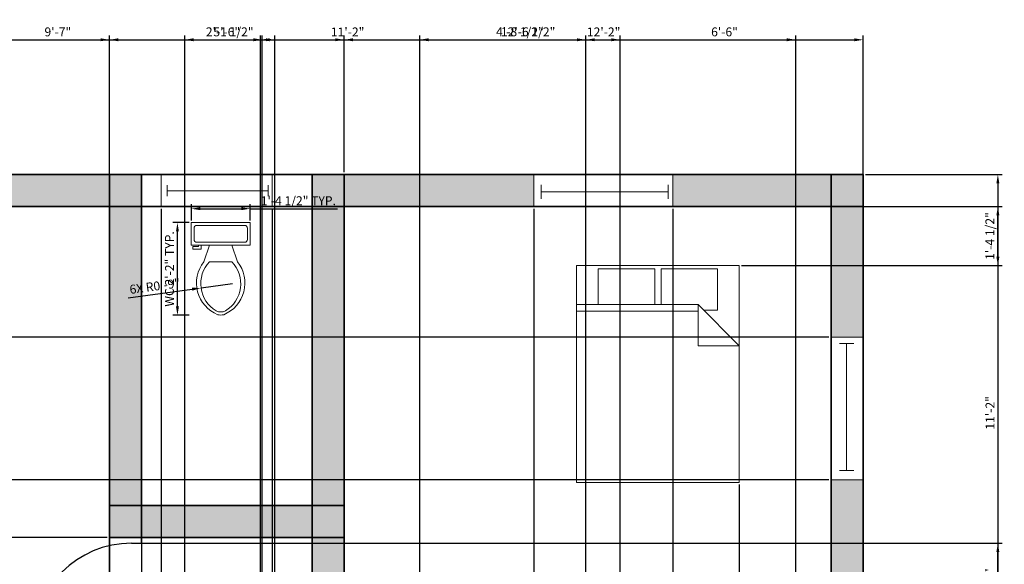
# Model space of a CAD drawing. Units: millimetres. Extents: x 2856 to 3283, y 634 to 1474.
# Tile 8 of 8: x 3006 to 3283, y 1321 to 1474. Entities that reach past the tile are written whole.
import ezdxf

# ---------------------------------------------------------------- set-up
doc = ezdxf.new("R2010")
doc.units = ezdxf.units.MM
for name, color, linetype, lineweight in [('A-ANNO-DIMS', 90, 'Continuous', 18), ('A-FLOR-FIXT', 140, 'Continuous', 18), ('A-WALL-PATT', 2, 'Continuous', 13), ('doors', 10, 'Continuous', 25), ('furniture', 140, 'Continuous', 18), ('walls', 50, 'Continuous', 35), ('windows', 30, 'Continuous', 18)]:
    doc.layers.add(name, color=color, linetype=linetype, lineweight=lineweight)
doc.styles.get("Standard").update_dxf_attribs({"font": 'arial.ttf'})
doc.dimstyles.new('ISO-25', dxfattribs={"dimtxt": 2.5, "dimasz": 2.5, "dimexe": 1.25, "dimexo": 0.625, "dimtad": 1, "dimdec": 0, "dimlunit": 3, "dimtxsty": 'Standard', "dimcen": 2.5, "dimadec": 0, "dimazin": 0, "dimtfac": 1, "dimtdec": 0, "dimtmove": 0, "dimatfit": 3, "dimfxl": 1, "dimarcsym": 0})

# ---------------------------------------------------------------- blocks, each defined once
blk = doc.blocks.new('*U3')
for p, q in [((0, 0), (0, -6)), ((40, 0), (40, -6))]:
    blk.add_line(p, q)
blk.add_lwpolyline([(0, 0), (0, 40), (1.75, 40), (1.75, 0)], close=True)
blk.add_arc((0, 0), 40, 0, 90)
blk = doc.blocks.new('*U5')
for p, q in [((0, 4), (0, 0)), ((36, 4), (36, 0)), ((0, 2), (36, 2))]:
    blk.add_line(p, q)
blk = doc.blocks.new('*U6')
for p, q in [((0, 4), (0, 0)), ((36, 4), (36, 0)), ((0, 2), (36, 2))]:
    blk.add_line(p, q)
blk = doc.blocks.new('Bed - Queen')
for p, q in [((0, -80.00003), (0, 0)), ((0, 0), (59.99999, 0)), ((59.99999, 0), (59.99999, -80.00003)), ((7.99999, -1.2), (28.79998, -1.2)), ((7.99999, -14.4), (7.99999, -1.2)), ((28.79998, -1.2), (28.79998, -14.4)), ((31.19999, -1.2), (51.99999, -1.2)), ((31.19999, -14.4), (31.19999, -1.2)), ((51.99999, -1.2), (51.99999, -16.4)), ((0, -14.4), (44.8, -14.4)), ((59.99999, -29.6), (44.8, -14.4)), ((44.8, -14.4), (44.8, -29.6)), ((44.8, -16.8), (0, -16.8)), ((51.99999, -16.4), (46.79936, -16.4)), ((44.8, -29.6), (59.99999, -29.6)), ((59.99999, -80.00003), (0, -80.00003))]:
    blk.add_line(p, q)
blk = doc.blocks.new('Toilet - top')
for p, q in [((9.5, -6), (9.5, -2)), ((-10, -8.5), (-8, -8.5)), ((-10, -9.5), (-10, -8.5)), ((-7, -9.5), (-10, -9.5)), ((-8, -8.5), (-8, -8)), ((-7, -8), (-7, -9.5)), ((-4, -8), (-6, -14)), ((4, -8), (6, -14)), ((4, -14), (-4, -14))]:
    blk.add_line(p, q)
blk.add_lwpolyline([(10.5, -8), (10.5, 0), (-10.5, 0), (-10.5, -8)], close=True)
for points in [[(-9.5, -2), (-9.5, -6)], [(8.5, -1), (-8.5, -1)], [(-8.5, -7), (8.5, -7)]]:
    blk.add_lwpolyline(points)
for centre, radius, start, end in [((-8.62, -1.88), 0.884, 81.8699, 188.1301), ((8.62, -1.88), 0.884, 351.8699, 98.1301), ((-8.62, -6.12), 0.884, 171.8699, 278.1301), ((8.62, -6.12), 0.884, 261.8699, 8.1301), ((3.52, -21.58), 12.17, 141.4691, 247.9714), ((4.2, -21.82), 11.33, 136.3677, 238.9468), ((-3.52, -21.58), 12.17, 292.0284, 38.5307), ((-4.2, -21.82), 11.33, 301.053, 43.6321), ((0, -27.88), 4, 245.7318, 294.2682), ((0, -29), 4, 254.8605, 285.1395)]:
    blk.add_arc(centre, radius, start, end)
blk = doc.blocks.new('*D20')
at = {"layer": 'A-ANNO-DIMS', "color": 0, "lineweight": -2, "transparency": 16777216}
for p, q in [((3053.58, 1417.43), (3049.05, 1417.43)), ((3050.3, 1393.88), (3050.3, 1414.93)), ((3053.58, 1391.38), (3049.05, 1391.38))]:
    blk.add_line(p, q, dxfattribs=at)
at = {"layer": 'A-ANNO-DIMS', "color": 0, "transparency": 16777216}
for points in [[(3049.88, 1414.93), (3050.72, 1414.93), (3050.3, 1417.43)], [(3049.88, 1393.88), (3050.72, 1393.88), (3050.3, 1391.38)]]:
    blk.add_solid(points, dxfattribs=at)
at = {"layer": 'Defpoints', "color": 0, "transparency": 16777216}
for p in [(3050.3, 1417.43), (3054.21, 1417.43), (3054.21, 1391.38)]:
    blk.add_point(p, dxfattribs=at)
at = {"layer": 'A-ANNO-DIMS', "color": 0, "transparency": 16777216, "insert": (3048.38, 1404.4), "char_height": 2.5, "attachment_point": 5, "rotation": 90}
blk.add_mtext('WC 2\'-2" TYP.', dxfattribs=at)
blk = doc.blocks.new('*D21')
at = {"layer": 'A-ANNO-DIMS', "color": 0, "lineweight": -2, "transparency": 16777216}
for p, q in [((3054.21, 1418.05), (3054.21, 1422.58)), ((3056.71, 1421.33), (3068.26, 1421.33)), ((3070.76, 1418.05), (3070.76, 1422.58)), ((3070.76, 1421.33), (3095.34, 1421.33))]:
    blk.add_line(p, q, dxfattribs=at)
at = {"layer": 'A-ANNO-DIMS', "color": 0, "transparency": 16777216}
for points in [[(3056.71, 1421.75), (3056.71, 1420.92), (3054.21, 1421.33)], [(3068.26, 1421.75), (3068.26, 1420.92), (3070.76, 1421.33)]]:
    blk.add_solid(points, dxfattribs=at)
at = {"layer": 'Defpoints', "color": 0, "transparency": 16777216}
for p in [(3070.76, 1421.33), (3054.21, 1417.43), (3070.76, 1417.43)]:
    blk.add_point(p, dxfattribs=at)
at = {"layer": 'A-ANNO-DIMS', "color": 0, "transparency": 16777216, "insert": (3084.3, 1423.25), "char_height": 2.5, "attachment_point": 5}
blk.add_mtext('1\'-4 1/2" TYP.', dxfattribs=at)
blk = doc.blocks.new('*D33')
at = {"layer": 'A-ANNO-DIMS', "color": 0, "lineweight": -2, "transparency": 16777216}
for p, q in [((3073.7, 1014.05), (3073.7, 1470.06)), ((3076.2, 1468.81), (3221.68, 1468.81)), ((3224.18, 1014.05), (3224.18, 1470.06))]:
    blk.add_line(p, q, dxfattribs=at)
at = {"layer": 'A-ANNO-DIMS', "color": 0, "transparency": 16777216}
for points in [[(3076.2, 1469.23), (3076.2, 1468.4), (3073.7, 1468.81)], [(3221.68, 1469.23), (3221.68, 1468.4), (3224.18, 1468.81)]]:
    blk.add_solid(points, dxfattribs=at)
at = {"layer": 'Defpoints', "color": 0, "transparency": 16777216}
for p in [(3224.18, 1468.81), (3073.7, 1013.42), (3224.18, 1013.42)]:
    blk.add_point(p, dxfattribs=at)
at = {"layer": 'A-ANNO-DIMS', "color": 0, "transparency": 16777216, "insert": (3148.94, 1470.73), "char_height": 2.5, "attachment_point": 5}
blk.add_mtext('12\'-6 1/2"', dxfattribs=at)
blk = doc.blocks.new('*D40')
at = {"layer": 'A-ANNO-DIMS', "color": 0, "lineweight": -2, "transparency": 16777216}
for p, q in [((3118.44, 913.07), (3118.44, 1470.06)), ((3120.94, 1468.81), (3172.32, 1468.81)), ((3174.82, 914.65), (3174.82, 1470.06))]:
    blk.add_line(p, q, dxfattribs=at)
at = {"layer": 'A-ANNO-DIMS', "color": 0, "transparency": 16777216}
for points in [[(3120.94, 1469.23), (3120.94, 1468.4), (3118.44, 1468.81)], [(3172.32, 1469.23), (3172.32, 1468.4), (3174.82, 1468.81)]]:
    blk.add_solid(points, dxfattribs=at)
at = {"layer": 'Defpoints', "color": 0, "transparency": 16777216}
for p in [(3174.82, 1468.81), (3174.82, 914.03), (3118.44, 912.44)]:
    blk.add_point(p, dxfattribs=at)
at = {"layer": 'A-ANNO-DIMS', "color": 0, "transparency": 16777216, "insert": (3146.63, 1470.73), "char_height": 2.5, "attachment_point": 5}
blk.add_mtext('4\'-8 1/2"', dxfattribs=at)
blk = doc.blocks.new('*D43')
at = {"layer": 'A-ANNO-DIMS', "color": 0, "lineweight": -2, "transparency": 16777216}
for p, q in [((3052.34, 800.56), (3052.34, 1470.06)), ((3054.84, 1468.81), (3075.18, 1468.81)), ((3077.68, 819.72), (3077.68, 1470.06))]:
    blk.add_line(p, q, dxfattribs=at)
at = {"layer": 'A-ANNO-DIMS', "color": 0, "transparency": 16777216}
for points in [[(3054.84, 1469.23), (3054.84, 1468.4), (3052.34, 1468.81)], [(3075.18, 1469.23), (3075.18, 1468.4), (3077.68, 1468.81)]]:
    blk.add_solid(points, dxfattribs=at)
at = {"layer": 'Defpoints', "color": 0, "transparency": 16777216}
for p in [(3077.68, 1468.81), (3077.68, 819.09), (3052.34, 799.94)]:
    blk.add_point(p, dxfattribs=at)
at = {"layer": 'A-ANNO-DIMS', "color": 0, "transparency": 16777216, "insert": (3065.01, 1470.73), "char_height": 2.5, "attachment_point": 5}
blk.add_mtext('2\'-1 1/2"', dxfattribs=at)
blk = doc.blocks.new('*D44')
at = {"layer": 'A-ANNO-DIMS', "color": 0, "lineweight": -2, "transparency": 16777216}
for p, q in [((2899.17, 1431.56), (2899.17, 1470.06)), ((2901.67, 1468.81), (3028.67, 1468.81)), ((3031.17, 1431.56), (3031.17, 1470.06))]:
    blk.add_line(p, q, dxfattribs=at)
at = {"layer": 'A-ANNO-DIMS', "color": 0, "transparency": 16777216}
for points in [[(2901.67, 1469.23), (2901.67, 1468.4), (2899.17, 1468.81)], [(3028.67, 1469.23), (3028.67, 1468.4), (3031.17, 1468.81)]]:
    blk.add_solid(points, dxfattribs=at)
at = {"layer": 'Defpoints', "color": 0, "transparency": 16777216}
for p in [(3031.17, 1468.81), (2899.17, 1430.94), (3031.17, 1430.94)]:
    blk.add_point(p, dxfattribs=at)
at = {"layer": 'A-ANNO-DIMS', "color": 0, "transparency": 16777216, "insert": (2965.17, 1470.71), "char_height": 2.5, "attachment_point": 5}
blk.add_mtext('11\'-0"', dxfattribs=at)
blk = doc.blocks.new('*D45')
at = {"layer": 'A-ANNO-DIMS', "color": 0, "lineweight": -2, "transparency": 16777216}
for p, q in [((3031.17, 1431.56), (3031.17, 1470.06)), ((3033.67, 1468.81), (3094.67, 1468.81)), ((3097.17, 1431.56), (3097.17, 1470.06))]:
    blk.add_line(p, q, dxfattribs=at)
at = {"layer": 'A-ANNO-DIMS', "color": 0, "transparency": 16777216}
for points in [[(3033.67, 1469.23), (3033.67, 1468.4), (3031.17, 1468.81)], [(3094.67, 1469.23), (3094.67, 1468.4), (3097.17, 1468.81)]]:
    blk.add_solid(points, dxfattribs=at)
at = {"layer": 'Defpoints', "color": 0, "transparency": 16777216}
for p in [(3097.17, 1468.81), (3031.17, 1430.94), (3097.17, 1430.94)]:
    blk.add_point(p, dxfattribs=at)
at = {"layer": 'A-ANNO-DIMS', "color": 0, "transparency": 16777216, "insert": (3064.17, 1470.71), "char_height": 2.5, "attachment_point": 5}
blk.add_mtext('5\'-6"', dxfattribs=at)
blk = doc.blocks.new('*D46')
at = {"layer": 'A-ANNO-DIMS', "color": 0, "lineweight": -2, "transparency": 16777216}
for p, q in [((3097.17, 1431.56), (3097.17, 1470.06)), ((3099.67, 1468.81), (3240.67, 1468.81)), ((3243.17, 1431.56), (3243.17, 1470.06))]:
    blk.add_line(p, q, dxfattribs=at)
at = {"layer": 'A-ANNO-DIMS', "color": 0, "transparency": 16777216}
for points in [[(3099.67, 1469.23), (3099.67, 1468.4), (3097.17, 1468.81)], [(3240.67, 1469.23), (3240.67, 1468.4), (3243.17, 1468.81)]]:
    blk.add_solid(points, dxfattribs=at)
at = {"layer": 'Defpoints', "color": 0, "transparency": 16777216}
for p in [(3243.17, 1468.81), (3097.17, 1430.94), (3243.17, 1430.94)]:
    blk.add_point(p, dxfattribs=at)
at = {"layer": 'A-ANNO-DIMS', "color": 0, "transparency": 16777216, "insert": (3170.17, 1470.69), "char_height": 2.5, "attachment_point": 5}
blk.add_mtext('12\'-2"', dxfattribs=at)
blk = doc.blocks.new('*D47')
at = {"layer": 'A-ANNO-DIMS', "color": 0, "lineweight": -2, "transparency": 16777216}
for p, q in [((3243.8, 1430.94), (3282.3, 1430.94)), ((3281.05, 1428.44), (3281.05, 1299.44)), ((3243.8, 1296.94), (3282.3, 1296.94))]:
    blk.add_line(p, q, dxfattribs=at)
at = {"layer": 'A-ANNO-DIMS', "color": 0, "transparency": 16777216}
for points in [[(3280.63, 1428.44), (3281.47, 1428.44), (3281.05, 1430.94)], [(3280.63, 1299.44), (3281.47, 1299.44), (3281.05, 1296.94)]]:
    blk.add_solid(points, dxfattribs=at)
at = {"layer": 'Defpoints', "color": 0, "transparency": 16777216}
for p in [(3243.17, 1430.94), (3243.17, 1296.94), (3281.05, 1296.94)]:
    blk.add_point(p, dxfattribs=at)
at = {"layer": 'A-ANNO-DIMS', "color": 0, "transparency": 16777216, "insert": (3279.17, 1363.94), "char_height": 2.5, "attachment_point": 5, "rotation": 90}
blk.add_mtext('11\'-2"', dxfattribs=at)
blk = doc.blocks.new('*D48')
at = {"layer": 'A-ANNO-DIMS', "color": 0, "lineweight": -2, "transparency": 16777216}
for p, q in [((3030.55, 1430.94), (2860.05, 1430.94)), ((2861.3, 1428.44), (2861.3, 1331.44)), ((3030.55, 1328.94), (2860.05, 1328.94))]:
    blk.add_line(p, q, dxfattribs=at)
at = {"layer": 'A-ANNO-DIMS', "color": 0, "transparency": 16777216}
for points in [[(2860.88, 1428.44), (2861.72, 1428.44), (2861.3, 1430.94)], [(2860.88, 1331.44), (2861.72, 1331.44), (2861.3, 1328.94)]]:
    blk.add_solid(points, dxfattribs=at)
at = {"layer": 'Defpoints', "color": 0, "transparency": 16777216}
for p in [(3031.17, 1430.94), (2861.3, 1328.94), (3031.17, 1328.94)]:
    blk.add_point(p, dxfattribs=at)
at = {"layer": 'A-ANNO-DIMS', "color": 0, "transparency": 16777216, "insert": (2859.4, 1379.94), "char_height": 2.5, "attachment_point": 5, "rotation": 90}
blk.add_mtext('8\'-6"', dxfattribs=at)
blk = doc.blocks.new('*D50')
at = {"layer": 'A-ANNO-DIMS', "color": 0, "lineweight": -2, "transparency": 16777216}
for p, q in [((3031.17, 1166.56), (3031.17, 1470.06)), ((3033.67, 1468.81), (3162.67, 1468.81)), ((3165.17, 1157.56), (3165.17, 1470.06))]:
    blk.add_line(p, q, dxfattribs=at)
at = {"layer": 'A-ANNO-DIMS', "color": 0, "transparency": 16777216}
for points in [[(3033.67, 1469.23), (3033.67, 1468.4), (3031.17, 1468.81)], [(3162.67, 1469.23), (3162.67, 1468.4), (3165.17, 1468.81)]]:
    blk.add_solid(points, dxfattribs=at)
at = {"layer": 'Defpoints', "color": 0, "transparency": 16777216}
for p in [(3165.17, 1468.81), (3031.17, 1165.94), (3165.17, 1156.94)]:
    blk.add_point(p, dxfattribs=at)
at = {"layer": 'A-ANNO-DIMS', "color": 0, "transparency": 16777216, "insert": (3098.17, 1470.69), "char_height": 2.5, "attachment_point": 5}
blk.add_mtext('11\'-2"', dxfattribs=at)
blk = doc.blocks.new('*D51')
at = {"layer": 'A-ANNO-DIMS', "color": 0, "lineweight": -2, "transparency": 16777216}
for p, q in [((3165.17, 1223.56), (3165.17, 1470.06)), ((3167.67, 1468.81), (3240.67, 1468.81)), ((3243.17, 1223.56), (3243.17, 1470.06))]:
    blk.add_line(p, q, dxfattribs=at)
at = {"layer": 'A-ANNO-DIMS', "color": 0, "transparency": 16777216}
for points in [[(3167.67, 1469.23), (3167.67, 1468.4), (3165.17, 1468.81)], [(3240.67, 1469.23), (3240.67, 1468.4), (3243.17, 1468.81)]]:
    blk.add_solid(points, dxfattribs=at)
at = {"layer": 'Defpoints', "color": 0, "transparency": 16777216}
for p in [(3243.17, 1468.81), (3165.17, 1222.94), (3243.17, 1222.94)]:
    blk.add_point(p, dxfattribs=at)
at = {"layer": 'A-ANNO-DIMS', "color": 0, "transparency": 16777216, "insert": (3204.17, 1470.71), "char_height": 2.5, "attachment_point": 5}
blk.add_mtext('6\'-6"', dxfattribs=at)
blk = doc.blocks.new('*D59')
at = {"layer": 'A-ANNO-DIMS', "color": 0, "lineweight": -2, "transparency": 16777216}
for p, q in [((2959.17, 1117.56), (2959.17, 1470.06)), ((2961.67, 1468.81), (3071.67, 1468.81)), ((3074.17, 1117.56), (3074.17, 1470.06))]:
    blk.add_line(p, q, dxfattribs=at)
at = {"layer": 'A-ANNO-DIMS', "color": 0, "transparency": 16777216}
for points in [[(2961.67, 1469.23), (2961.67, 1468.4), (2959.17, 1468.81)], [(3071.67, 1469.23), (3071.67, 1468.4), (3074.17, 1468.81)]]:
    blk.add_solid(points, dxfattribs=at)
at = {"layer": 'Defpoints', "color": 0, "transparency": 16777216}
for p in [(3074.17, 1468.81), (2959.17, 1116.94), (3074.17, 1116.94)]:
    blk.add_point(p, dxfattribs=at)
at = {"layer": 'A-ANNO-DIMS', "color": 0, "transparency": 16777216, "insert": (3016.67, 1470.71), "char_height": 2.5, "attachment_point": 5}
blk.add_mtext('9\'-7"', dxfattribs=at)
blk = doc.blocks.new('*D61')
at = {"layer": 'A-ANNO-DIMS', "color": 0, "lineweight": -2, "transparency": 16777216}
for p, q in [((3031.17, 1430.31), (3031.17, 634.81)), ((3040.17, 1430.31), (3040.17, 634.81)), ((3033.67, 636.06), (3037.67, 636.06))]:
    blk.add_line(p, q, dxfattribs=at)
at = {"layer": 'A-ANNO-DIMS', "color": 0, "transparency": 16777216}
for points in [[(3033.67, 636.48), (3033.67, 635.65), (3031.17, 636.06)], [(3037.67, 636.48), (3037.67, 635.65), (3040.17, 636.06)]]:
    blk.add_solid(points, dxfattribs=at)
at = {"layer": 'Defpoints', "color": 0, "transparency": 16777216}
for p in [(3031.17, 1430.94), (3040.17, 1430.94), (3040.17, 636.06)]:
    blk.add_point(p, dxfattribs=at)
at = {"layer": 'A-ANNO-DIMS', "color": 0, "transparency": 16777216, "insert": (3035.67, 637.96), "char_height": 2.5, "attachment_point": 5}
blk.add_mtext('0\'-9"', dxfattribs=at)
blk = doc.blocks.new('*D68')
at = {"layer": 'A-ANNO-DIMS', "color": 0, "lineweight": -2, "transparency": 16777216}
for p, q in [((3040.8, 1327.29), (3282.3, 1327.29)), ((3281.05, 1302.28), (3281.05, 1324.79)), ((3040.8, 1299.78), (3282.3, 1299.78))]:
    blk.add_line(p, q, dxfattribs=at)
at = {"layer": 'A-ANNO-DIMS', "color": 0, "transparency": 16777216}
for points in [[(3280.63, 1324.79), (3281.47, 1324.79), (3281.05, 1327.29)], [(3280.63, 1302.28), (3281.47, 1302.28), (3281.05, 1299.78)]]:
    blk.add_solid(points, dxfattribs=at)
at = {"layer": 'Defpoints', "color": 0, "transparency": 16777216}
for p in [(3040.17, 1327.29), (3281.05, 1327.29), (3040.17, 1299.78)]:
    blk.add_point(p, dxfattribs=at)
at = {"layer": 'A-ANNO-DIMS', "color": 0, "transparency": 16777216, "insert": (3279.13, 1313.53), "char_height": 2.5, "attachment_point": 5, "rotation": 90}
blk.add_mtext('2\'-3 1/2"', dxfattribs=at)
blk = doc.blocks.new('*D70')
at = {"layer": 'A-ANNO-DIMS', "color": 0, "lineweight": -2, "transparency": 16777216}
for p, q in [((3045.69, 1421.31), (3045.69, 634.81)), ((3076.97, 1421.31), (3076.97, 634.81)), ((3048.19, 636.06), (3074.47, 636.06))]:
    blk.add_line(p, q, dxfattribs=at)
at = {"layer": 'A-ANNO-DIMS', "color": 0, "transparency": 16777216}
for points in [[(3048.19, 636.48), (3048.19, 635.65), (3045.69, 636.06)], [(3074.47, 636.48), (3074.47, 635.65), (3076.97, 636.06)]]:
    blk.add_solid(points, dxfattribs=at)
at = {"layer": 'Defpoints', "color": 0, "transparency": 16777216}
for p in [(3045.69, 1421.94), (3076.97, 1421.94), (3076.97, 636.06)]:
    blk.add_point(p, dxfattribs=at)
at = {"layer": 'A-ANNO-DIMS', "color": 0, "transparency": 16777216, "insert": (3061.33, 637.98), "char_height": 2.5, "attachment_point": 5}
blk.add_mtext('2\'-7 1/2"', dxfattribs=at)
blk = doc.blocks.new('*D71')
at = {"layer": 'A-ANNO-DIMS', "color": 0, "lineweight": -2, "transparency": 16777216}
for p, q in [((3150.5, 1421.31), (3150.5, 634.81)), ((3189.65, 1421.31), (3189.65, 634.81)), ((3153, 636.06), (3187.15, 636.06))]:
    blk.add_line(p, q, dxfattribs=at)
at = {"layer": 'A-ANNO-DIMS', "color": 0, "transparency": 16777216}
for points in [[(3153, 636.48), (3153, 635.65), (3150.5, 636.06)], [(3187.15, 636.48), (3187.15, 635.65), (3189.65, 636.06)]]:
    blk.add_solid(points, dxfattribs=at)
at = {"layer": 'Defpoints', "color": 0, "transparency": 16777216}
for p in [(3150.5, 1421.94), (3189.65, 1421.94), (3189.65, 636.06)]:
    blk.add_point(p, dxfattribs=at)
at = {"layer": 'A-ANNO-DIMS', "color": 0, "transparency": 16777216, "insert": (3170.07, 637.97), "char_height": 2.5, "attachment_point": 5}
blk.add_mtext('3\'-3"', dxfattribs=at)
blk = doc.blocks.new('*D72')
at = {"layer": 'A-ANNO-DIMS', "color": 0, "lineweight": -2, "transparency": 16777216}
for p, q in [((3233.55, 1385.21), (2860.05, 1385.21)), ((2861.3, 1347.66), (2861.3, 1382.71)), ((3233.55, 1345.16), (2860.05, 1345.16))]:
    blk.add_line(p, q, dxfattribs=at)
at = {"layer": 'A-ANNO-DIMS', "color": 0, "transparency": 16777216}
for points in [[(2860.88, 1382.71), (2861.72, 1382.71), (2861.3, 1385.21)], [(2860.88, 1347.66), (2861.72, 1347.66), (2861.3, 1345.16)]]:
    blk.add_solid(points, dxfattribs=at)
at = {"layer": 'Defpoints', "color": 0, "transparency": 16777216}
for p in [(2861.3, 1385.21), (3234.17, 1385.21), (3234.17, 1345.16)]:
    blk.add_point(p, dxfattribs=at)
at = {"layer": 'A-ANNO-DIMS', "color": 0, "transparency": 16777216, "insert": (2859.4, 1365.19), "char_height": 2.5, "attachment_point": 5, "rotation": 90}
blk.add_mtext('3\'-4"', dxfattribs=at)
blk = doc.blocks.new('*D77')
at = {"layer": 'A-ANNO-DIMS', "color": 0, "lineweight": -2, "transparency": 16777216}
for p, q in [((3097.17, 1430.31), (3097.17, 634.81)), ((3150.5, 1421.31), (3150.5, 634.81)), ((3099.67, 636.06), (3148, 636.06))]:
    blk.add_line(p, q, dxfattribs=at)
at = {"layer": 'A-ANNO-DIMS', "color": 0, "transparency": 16777216}
for points in [[(3099.67, 636.48), (3099.67, 635.65), (3097.17, 636.06)], [(3148, 636.48), (3148, 635.65), (3150.5, 636.06)]]:
    blk.add_solid(points, dxfattribs=at)
at = {"layer": 'Defpoints', "color": 0, "transparency": 16777216}
for p in [(3097.17, 1430.94), (3150.5, 1421.94), (3150.5, 636.06)]:
    blk.add_point(p, dxfattribs=at)
at = {"layer": 'A-ANNO-DIMS', "color": 0, "transparency": 16777216, "insert": (3123.84, 637.98), "char_height": 2.5, "attachment_point": 5}
blk.add_mtext('4\'-5 1/2"', dxfattribs=at)
blk = doc.blocks.new('*D78')
at = {"layer": 'A-ANNO-DIMS', "color": 0, "lineweight": -2, "transparency": 16777216}
for p, q in [((3233.55, 1430.94), (2860.05, 1430.94)), ((2861.3, 1387.71), (2861.3, 1428.44)), ((3233.55, 1385.21), (2860.05, 1385.21))]:
    blk.add_line(p, q, dxfattribs=at)
at = {"layer": 'A-ANNO-DIMS', "color": 0, "transparency": 16777216}
for points in [[(2860.88, 1428.44), (2861.72, 1428.44), (2861.3, 1430.94)], [(2860.88, 1387.71), (2861.72, 1387.71), (2861.3, 1385.21)]]:
    blk.add_solid(points, dxfattribs=at)
at = {"layer": 'Defpoints', "color": 0, "transparency": 16777216}
for p in [(2861.3, 1430.94), (3234.17, 1430.94), (3234.17, 1385.21)]:
    blk.add_point(p, dxfattribs=at)
at = {"layer": 'A-ANNO-DIMS', "color": 0, "transparency": 16777216, "insert": (2859.38, 1408.08), "char_height": 2.5, "attachment_point": 5, "rotation": 90}
blk.add_mtext('3\'-9 1/2"', dxfattribs=at)
blk = doc.blocks.new('*D92')
at = {"layer": 'A-ANNO-DIMS', "color": 0, "lineweight": -2, "transparency": 16777216}
for p, q in [((3208.3, 1343.77), (3208.3, 634.81)), ((3234.17, 1344.54), (3234.17, 634.81)), ((3210.8, 636.06), (3231.67, 636.06))]:
    blk.add_line(p, q, dxfattribs=at)
at = {"layer": 'A-ANNO-DIMS', "color": 0, "transparency": 16777216}
for points in [[(3210.8, 636.48), (3210.8, 635.65), (3208.3, 636.06)], [(3231.67, 636.48), (3231.67, 635.65), (3234.17, 636.06)]]:
    blk.add_solid(points, dxfattribs=at)
at = {"layer": 'Defpoints', "color": 0, "transparency": 16777216}
for p in [(3208.3, 1344.39), (3234.17, 1345.16), (3234.17, 636.06)]:
    blk.add_point(p, dxfattribs=at)
at = {"layer": 'A-ANNO-DIMS', "color": 0, "transparency": 16777216, "insert": (3221.24, 637.94), "char_height": 2.5, "attachment_point": 5}
blk.add_mtext('2\'-2"', dxfattribs=at)
blk = doc.blocks.new('*D93')
at = {"layer": 'A-ANNO-DIMS', "color": 0, "lineweight": -2, "transparency": 16777216}
for p, q in [((3190.27, 1421.94), (3282.3, 1421.94)), ((3281.05, 1407.85), (3281.05, 1419.44)), ((3208.93, 1405.35), (3282.3, 1405.35))]:
    blk.add_line(p, q, dxfattribs=at)
at = {"layer": 'A-ANNO-DIMS', "color": 0, "transparency": 16777216}
for points in [[(3280.63, 1419.44), (3281.47, 1419.44), (3281.05, 1421.94)], [(3280.63, 1407.85), (3281.47, 1407.85), (3281.05, 1405.35)]]:
    blk.add_solid(points, dxfattribs=at)
at = {"layer": 'Defpoints', "color": 0, "transparency": 16777216}
for p in [(3189.65, 1421.94), (3281.05, 1421.94), (3208.3, 1405.35)]:
    blk.add_point(p, dxfattribs=at)
at = {"layer": 'A-ANNO-DIMS', "color": 0, "transparency": 16777216, "insert": (3279.13, 1413.65), "char_height": 2.5, "attachment_point": 5, "rotation": 90}
blk.add_mtext('1\'-4 1/2"', dxfattribs=at)
blk = doc.blocks.new('*D98')
at = {"layer": 'A-ANNO-DIMS', "color": 0, "lineweight": -2, "transparency": 16777216}
for p, q in [((3088.17, 1430.31), (3088.17, 634.81)), ((3076.97, 1421.31), (3076.97, 634.81)), ((3079.47, 636.06), (3085.67, 636.06))]:
    blk.add_line(p, q, dxfattribs=at)
at = {"layer": 'A-ANNO-DIMS', "color": 0, "transparency": 16777216}
for points in [[(3079.47, 636.48), (3079.47, 635.65), (3076.97, 636.06)], [(3085.67, 636.48), (3085.67, 635.65), (3088.17, 636.06)]]:
    blk.add_solid(points, dxfattribs=at)
at = {"layer": 'Defpoints', "color": 0, "transparency": 16777216}
for p in [(3088.17, 1430.94), (3076.97, 1421.94), (3088.17, 636.06)]:
    blk.add_point(p, dxfattribs=at)
at = {"layer": 'A-ANNO-DIMS', "color": 0, "transparency": 16777216, "insert": (3082.57, 637.96), "char_height": 2.5, "attachment_point": 5}
blk.add_mtext('0\'-11"', dxfattribs=at)
blk = doc.blocks.new('*D102')
at = {"layer": 'A-ANNO-DIMS', "color": 0, "lineweight": -2, "transparency": 16777216}
for p, q in [((3036.45, 1396.29), (3054.47, 1398.71)), ((3065.79, 1400.23), (3056.94, 1399.04))]:
    blk.add_line(p, q, dxfattribs=at)
at = {"layer": 'A-ANNO-DIMS', "color": 0, "transparency": 16777216}
blk.add_solid([(3054.41, 1399.12), (3054.52, 1398.3), (3056.94, 1399.04)], dxfattribs=at)
at = {"layer": 'Defpoints', "color": 0, "transparency": 16777216}
for p in [(3056.94, 1399.04), (3065.79, 1400.23)]:
    blk.add_point(p, dxfattribs=at)
at = {"layer": 'A-ANNO-DIMS', "color": 0, "transparency": 16777216, "insert": (3043.97, 1399.22), "char_height": 2.5, "attachment_point": 5, "rotation": 7.6594}
blk.add_mtext('6X R0\'-9"', dxfattribs=at)

msp = doc.modelspace()

# ---------------------------------------------------------------- hatches: boundary and pattern name
at = {"layer": 'A-WALL-PATT'}
h = msp.add_hatch(color=256, dxfattribs=at)
h.dxf.hatch_style = 1
h.paths.add_polyline_path([(2908.17, 1430.94), (2899.17, 1430.94), (2899.17, 1421.94), (2908.17, 1421.94)])
h.paths.add_polyline_path([(2908.17, 1421.94), (2899.17, 1421.94), (2899.17, 1296.94), (2908.17, 1296.94)])
h.paths.add_polyline_path([(2940.27, 1430.94), (2908.17, 1430.94), (2908.17, 1421.94), (2940.27, 1421.94)])
h.paths.add_polyline_path([(3031.17, 1430.94), (2982.35, 1430.94), (2982.35, 1421.94), (3031.17, 1421.94)])
h.paths.add_polyline_path([(3150.5, 1430.94), (3097.17, 1430.94), (3097.17, 1421.94), (3150.5, 1421.94)])
h.paths.add_polyline_path([(3097.17, 1430.94), (3088.17, 1430.94), (3088.17, 1421.94), (3097.17, 1421.94)])
h.paths.add_polyline_path([(3097.17, 1421.94), (3088.17, 1421.94), (3088.17, 1337.94), (3097.17, 1337.94)])
h.paths.add_polyline_path([(3088.17, 1337.94), (3040.17, 1337.94), (3040.17, 1328.94), (3088.17, 1328.94)])
h.paths.add_polyline_path([(3097.17, 1337.94), (3088.17, 1337.94), (3088.17, 1328.94), (3097.17, 1328.94)])
h.paths.add_polyline_path([(3097.17, 1328.94), (3088.17, 1328.94), (3088.17, 1296.94), (3097.17, 1296.94)])
h.paths.add_polyline_path([(3097.17, 1296.94), (3088.17, 1296.94), (3088.17, 1287.94), (3097.17, 1287.94)])
h.paths.add_polyline_path([(3040.17, 1421.94), (3031.17, 1421.94), (3031.17, 1337.94), (3040.17, 1337.94)])
h.paths.add_polyline_path([(3040.17, 1337.94), (3031.17, 1337.94), (3031.17, 1328.94), (3040.17, 1328.94)])
h.paths.add_polyline_path([(3040.17, 1430.94), (3031.17, 1430.94), (3031.17, 1421.94), (3040.17, 1421.94)])
h.paths.add_polyline_path([(3243.17, 1421.94), (3234.17, 1421.94), (3234.17, 1385.21), (3243.17, 1385.21)])
h.paths.add_polyline_path([(3243.17, 1430.94), (3234.17, 1430.94), (3234.17, 1421.94), (3243.17, 1421.94)])
h.paths.add_polyline_path([(3234.17, 1430.94), (3189.65, 1430.94), (3189.65, 1421.94), (3234.17, 1421.94)])
h.paths.add_polyline_path([(3243.17, 1345.16), (3234.17, 1345.16), (3234.17, 1296.94), (3243.17, 1296.94)])
h.paths.add_polyline_path([(3234.17, 1296.94), (3128.45, 1296.94, -0.06768), (3129.44, 1289.59), (3129.44, 1287.94), (3234.17, 1287.94)])
h.paths.add_polyline_path([(3031.17, 1296.94), (2908.17, 1296.94), (2908.17, 1287.94), (3031.17, 1287.94)])
h.paths.add_polyline_path([(3040.17, 1296.94), (3031.17, 1296.94), (3031.17, 1287.94), (3040.17, 1287.94)])
h.paths.add_polyline_path([(2908.17, 1296.94), (2899.17, 1296.94), (2899.17, 1287.94), (2908.17, 1287.94)])
h.paths.add_polyline_path([(2908.17, 1287.94), (2899.17, 1287.94), (2899.17, 1235.12), (2908.17, 1235.12)])
h.paths.add_polyline_path([(3040.17, 1287.94), (3031.17, 1287.94), (3031.17, 1165.94), (3040.17, 1165.94)])
h.paths.add_polyline_path([(3165.17, 1165.94), (3040.17, 1165.94), (3040.17, 1156.94), (3165.17, 1156.94)])
h.paths.add_polyline_path([(3040.17, 1165.94), (3031.17, 1165.94), (3031.17, 1156.94), (3040.17, 1156.94)])
h.paths.add_polyline_path([(3040.17, 1156.94), (3031.17, 1156.94), (3031.17, 1147.75, -0.068303), (3038.59, 1148.77), (3040.17, 1148.77)])
h.paths.add_polyline_path([(3174.17, 1197.55), (3166.11, 1197.55), (3165.17, 1197.55), (3165.17, 1165.94), (3174.17, 1165.94)])
h.paths.add_polyline_path([(3174.17, 1165.94), (3165.17, 1165.94), (3165.17, 1156.94), (3174.17, 1156.94)])
h.paths.add_polyline_path([(3234.17, 1165.94), (3174.17, 1165.94), (3174.17, 1156.94), (3234.17, 1156.94)])
h.paths.add_polyline_path([(3243.17, 1165.94), (3234.17, 1165.94), (3234.17, 1156.94), (3243.17, 1156.94)])
h.paths.add_polyline_path([(3243.17, 1172.31), (3234.17, 1172.31), (3234.17, 1165.94), (3243.17, 1165.94)])
h.paths.add_polyline_path([(3243.17, 1222.94), (3234.17, 1222.94), (3234.17, 1213.94), (3243.17, 1213.94)])
h.paths.add_polyline_path([(3234.17, 1222.94), (3174.17, 1222.94), (3174.17, 1213.94), (3234.17, 1213.94)])
h.paths.add_polyline_path([(3174.17, 1222.94), (3165.17, 1222.94), (3165.17, 1213.94), (3174.17, 1213.94)])
h.paths.add_polyline_path([(3174.17, 1270.54, -0.139319), (3166.75, 1268.43), (3165.17, 1268.43), (3165.17, 1222.94), (3174.17, 1222.94)])
h.paths.add_polyline_path([(3243.17, 1243.94), (3234.17, 1243.94), (3234.17, 1222.94), (3243.17, 1222.94)])
h.paths.add_polyline_path([(3243.17, 1213.94), (3234.17, 1213.94), (3234.17, 1203.68), (3243.17, 1203.68)])
h.paths.add_polyline_path([(3174.17, 1213.94), (3165.17, 1213.94), (3165.17, 1210.62), (3166.11, 1210.62, -0.16772), (3174.17, 1207.84)])
h.paths.add_polyline_path([(3243.17, 1296.94), (3234.17, 1296.94), (3234.17, 1287.94), (3243.17, 1287.94)])
h.paths.add_polyline_path([(3243.17, 1287.94), (3234.17, 1287.94), (3234.17, 1276.76), (3243.17, 1276.76)])
h.paths.add_polyline_path([(3174.17, 1287.94), (3165.17, 1287.94), (3165.17, 1282.56), (3166.75, 1282.56), (3174.17, 1282.56)])
h.paths.add_polyline_path([(2908.17, 1190.69), (2899.17, 1190.69), (2899.17, 1116.94), (2908.17, 1116.94)])
h.paths.add_polyline_path([(2908.17, 1107.94), (2899.17, 1107.94), (2899.17, 1058.94), (2908.17, 1058.94)])
h.paths.add_polyline_path([(2908.17, 1116.94), (2899.17, 1116.94), (2899.17, 1107.94), (2908.17, 1107.94)])
h.paths.add_polyline_path([(2959.17, 1107.94), (2950.17, 1107.94), (2950.17, 1058.94), (2959.17, 1058.94)])
h.paths.add_polyline_path([(2959.17, 1116.94), (2950.17, 1116.94), (2950.17, 1107.94), (2959.17, 1107.94)])
h.paths.add_polyline_path([(2950.17, 1116.94), (2908.17, 1116.94), (2908.17, 1107.94), (2950.17, 1107.94)])
h.paths.add_polyline_path([(3031.17, 1116.94), (2959.17, 1116.94), (2959.17, 1107.94), (3031.17, 1107.94)])
h.paths.add_polyline_path([(3074.17, 1116.94), (3065.17, 1116.94), (3065.17, 1107.94), (3074.17, 1107.94)])
h.paths.add_polyline_path([(3065.17, 1116.94), (3040.17, 1116.94), (3040.17, 1107.94), (3065.17, 1107.94)])
h.paths.add_polyline_path([(3040.17, 1116.94), (3031.17, 1116.94), (3031.17, 1107.94), (3040.17, 1107.94)])
h.paths.add_polyline_path([(3040.17, 1121.26), (3038.59, 1121.26), (3031.17, 1121.26), (3031.17, 1116.94), (3040.17, 1116.94)])
h.paths.add_polyline_path([(3074.17, 1107.94), (3065.17, 1107.94), (3065.17, 1058.94), (3074.17, 1058.94)])
h.paths.add_polyline_path([(3074.17, 1058.94), (3065.17, 1058.94), (3065.17, 1049.94), (3074.17, 1049.94)])
h.paths.add_polyline_path([(3065.17, 1058.94), (2975.4, 1058.94, -0.174756), (2978.69, 1049.94), (3065.17, 1049.94)])
h.paths.add_polyline_path([(2929.83, 1051.89), (2930.25, 1058.94), (2908.17, 1058.94), (2908.17, 1049.94), (2929.71, 1049.94)])
h.paths.add_polyline_path([(2908.17, 1058.94), (2899.17, 1058.94), (2899.17, 1049.94), (2908.17, 1049.94)])
h.paths.add_polyline_path([(2950.17, 1058.94), (2942.07, 1058.94, -0.146602), (2943.93, 1051.05), (2943.86, 1049.94), (2950.17, 1049.94)])
h.paths.add_polyline_path([(2959.17, 1058.94), (2950.17, 1058.94), (2950.17, 1049.94), (2959.17, 1049.94)])
h.paths.add_polyline_path([(2964.56, 1058.94), (2959.17, 1058.94), (2959.17, 1049.94), (2964.56, 1049.94)])
h.paths.add_polyline_path([(2908.17, 1049.94), (2899.17, 1049.94), (2899.17, 799.94), (2908.17, 799.94)])
h.paths.add_polyline_path([(3234.17, 1058.94), (3074.17, 1058.94), (3074.17, 1049.94), (3234.17, 1049.94)])
h.paths.add_polyline_path([(3243.17, 1156.94), (3234.17, 1156.94), (3234.17, 1058.94), (3243.17, 1058.94)])
h.paths.add_polyline_path([(3243.17, 1058.94), (3234.17, 1058.94), (3234.17, 1049.94), (3243.17, 1049.94)])
h.paths.add_polyline_path([(3243.17, 1049.94), (3234.17, 1049.94), (3234.17, 931.7), (3234.17, 799.94), (3243.17, 799.94), (3243.17, 931.7)])
h.paths.add_polyline_path([(2908.17, 790.94), (2899.17, 790.94), (2899.17, 682.94), (2908.17, 682.94)])
h.paths.add_polyline_path([(2908.17, 799.94), (2899.17, 799.94), (2899.17, 790.94), (2908.17, 790.94)])
h.paths.add_polyline_path([(3234.17, 799.94), (2908.17, 799.94), (2908.17, 790.94), (3234.17, 790.94)])
h.paths.add_polyline_path([(3243.17, 799.94), (3234.17, 799.94), (3234.17, 790.94), (3243.17, 790.94)])
h.paths.add_polyline_path([(3243.17, 790.94), (3234.17, 790.94), (3234.17, 682.94), (3243.17, 682.94)])
h.paths.add_polyline_path([(3234.17, 682.94), (2908.17, 682.94), (2908.17, 673.94), (3234.17, 673.94)])
h.paths.add_polyline_path([(3243.17, 682.94), (3234.17, 682.94), (3234.17, 673.94), (3243.17, 673.94)])
h.paths.add_polyline_path([(2908.17, 682.94), (2899.17, 682.94), (2899.17, 673.94), (2908.17, 673.94)])

# ---------------------------------------------------------------- linework, layer by layer
at = {"layer": 'walls'}
for p, q in [((2899.17, 1430.94), (3243.17, 1430.94)), ((3031.17, 1430.94), (3031.17, 1326.58)), ((3031.17, 1430.94), (3031.17, 1326.58)), ((3040.17, 1430.94), (3040.17, 1327.29)), ((3040.17, 1430.94), (3040.17, 1327.29)), ((3088.17, 1430.94), (3088.17, 1287.94)), ((3097.17, 1430.94), (3097.17, 1287.94)), ((3234.17, 1430.94), (3234.17, 1287.94)), ((3243.17, 1430.94), (3243.17, 1287.94)), ((2899.17, 1421.94), (3243.17, 1421.94)), ((3031.17, 1337.94), (3097.17, 1337.94)), ((3031.17, 1328.94), (3097.17, 1328.94))]:
    msp.add_line(p, q, dxfattribs=at)
at = {"layer": 'windows'}
for p, q in [((3045.69, 1421.94), (3045.69, 1430.94)), ((3076.97, 1421.94), (3076.97, 1430.94)), ((3150.5, 1430.94), (3150.5, 1421.94)), ((3189.65, 1430.94), (3189.65, 1421.94)), ((3234.17, 1385.21), (3243.17, 1385.21)), ((3243.17, 1345.16), (3234.17, 1345.16))]:
    msp.add_line(p, q, dxfattribs=at)

# ---------------------------------------------------------------- block references
at = {"layer": 'A-FLOR-FIXT', "xscale": 0.7880357630815594, "yscale": 0.7880357630815594, "zscale": 0.7880357630815594}
msp.add_blockref('Toilet - top', (3062.48, 1417.43), dxfattribs=at)
at = {"layer": 'doors', "xscale": 0.6877590013859352, "yscale": 0.6877590013859352, "zscale": 0.6877590013859352, "rotation": 90}
msp.add_blockref('*U3', (3037.35, 1299.78), dxfattribs=at)
at = {"layer": 'furniture', "xscale": 0.7619997142501188, "yscale": 0.7619997142501188, "zscale": 0.7619997142501188}
msp.add_blockref('Bed - Queen', (3162.58, 1405.35), dxfattribs=at)
at = {"layer": 'windows'}
for name, p, xscale, yscale, zscale in [('*U6', (3047.37, 1424.81), 0.7908534711778109, 0.7908534711778109, 0.7908534711778109), ('*U5', (3152.58, 1424.07), 0.9925939517092485, 0.9925939517092485, 0.9925939517092485)]:
    msp.add_blockref(name, p, dxfattribs=dict(at, xscale=xscale, yscale=yscale, zscale=zscale))
at = {"layer": 'windows', "xscale": 0.9925939517092485, "yscale": 0.9925939517092485, "zscale": 0.9925939517092485, "rotation": 90}
msp.add_blockref('*U5', (3240.5, 1347.71), dxfattribs=at)

# ---------------------------------------------------------------- dimensions: what is measured, and where the dimension line sits
at = {"layer": 'A-ANNO-DIMS'}
for base, p1, p2, picture, middle in [((3077.68, 1468.81), (3052.34, 799.94), (3077.68, 819.09), '*D43', (3065.01, 1470.73)), ((3224.18, 1468.81), (3073.7, 1013.42), (3224.18, 1013.42), '*D33', (3148.94, 1470.73)), ((3174.82, 1468.81), (3118.44, 912.44), (3174.82, 914.03), '*D40', (3146.63, 1470.73)), ((3031.17, 1468.81), (2899.17, 1430.94), (3031.17, 1430.94), '*D44', (2965.17, 1470.71)), ((3074.17, 1468.81), (2959.17, 1116.94), (3074.17, 1116.94), '*D59', (3016.67, 1470.71)), ((3097.17, 1468.81), (3031.17, 1430.94), (3097.17, 1430.94), '*D45', (3064.17, 1470.71)), ((3165.17, 1468.81), (3031.17, 1165.94), (3165.17, 1156.94), '*D50', (3098.17, 1470.69)), ((3243.17, 1468.81), (3097.17, 1430.94), (3243.17, 1430.94), '*D46', (3170.17, 1470.69)), ((3243.17, 1468.81), (3165.17, 1222.94), (3243.17, 1222.94), '*D51', (3204.17, 1470.71)), ((3040.17, 636.06), (3031.17, 1430.94), (3040.17, 1430.94), '*D61', (3035.67, 637.96)), ((3088.17, 636.06), (3076.97, 1421.94), (3088.17, 1430.94), '*D98', (3082.57, 637.96)), ((3150.5, 636.06), (3097.17, 1430.94), (3150.5, 1421.94), '*D77', (3123.84, 637.98)), ((3076.97, 636.06), (3045.69, 1421.94), (3076.97, 1421.94), '*D70', (3061.33, 637.98)), ((3189.6495, 636.0634), (3150.4985, 1421.9396), (3189.6495, 1421.9396), '*D71', (3170.074, 637.9657)), ((3234.17, 636.06), (3208.3, 1344.39), (3234.17, 1345.16), '*D92', (3221.24, 637.94))]:
    dim = msp.add_linear_dim(base=base, p1=p1, p2=p2, dimstyle='ISO-25', override={"dimdec": 1, "dimlfac": 1, "dimrnd": 0, "dimzin": 1, "dimdsep": 46, "dimlunit": 4, "dimfrac": 2}, dxfattribs=at)
    dim.commit()
    dim.dimension.update_dxf_attribs({"geometry": picture, "text_midpoint": middle})
for base, p1, p2, picture, middle in [((2861.3, 1430.94), (3234.17, 1385.21), (3234.17, 1430.94), '*D78', (2859.38, 1408.08)), ((2861.3, 1328.94), (3031.17, 1430.94), (3031.17, 1328.94), '*D48', (2859.4, 1379.94)), ((3281.05, 1296.94), (3243.17, 1430.94), (3243.17, 1296.94), '*D47', (3279.17, 1363.94)), ((3281.05, 1421.94), (3208.3, 1405.35), (3189.65, 1421.94), '*D93', (3279.13, 1413.65)), ((2861.3003, 1385.2147), (3234.1743, 1345.1601), (3234.1743, 1385.2147), '*D72', (2859.3981, 1365.1874)), ((3281.05, 1327.29), (3040.17, 1299.78), (3040.17, 1327.29), '*D68', (3279.13, 1313.53))]:
    dim = msp.add_linear_dim(base=base, p1=p1, p2=p2, angle=90, dimstyle='ISO-25', override={"dimdec": 1, "dimlfac": 1, "dimrnd": 0, "dimzin": 1, "dimdsep": 46, "dimlunit": 4, "dimfrac": 2}, dxfattribs=at)
    dim.commit()
    dim.dimension.update_dxf_attribs({"geometry": picture, "text_midpoint": middle})
dim = msp.add_linear_dim(base=(3070.7565, 1421.332), p1=(3054.2077, 1417.4258), p2=(3070.7565, 1417.4258), text='<> TYP.', dimstyle='ISO-25', override={"dimdec": 1, "dimlfac": 1, "dimrnd": 0, "dimzin": 1, "dimdsep": 46, "dimlunit": 4, "dimfrac": 2}, dxfattribs=at)
dim.commit()
dim.dimension.update_dxf_attribs({"geometry": '*D21', "text_midpoint": (3084.2959, 1423.2497)})
dim = msp.add_linear_dim(base=(3050.3015, 1417.4258), p1=(3054.2077, 1391.3842), p2=(3054.2077, 1417.4258), angle=90, text='WC <> TYP.', dimstyle='ISO-25', override={"dimdec": 1, "dimlfac": 1, "dimrnd": 0, "dimzin": 1, "dimdsep": 46, "dimlunit": 4, "dimfrac": 2}, dxfattribs=at)
dim.commit()
dim.dimension.update_dxf_attribs({"geometry": '*D20', "text_midpoint": (3048.3838, 1404.405)})
dim = msp.add_radius_dim(center=(3065.79, 1400.23), mpoint=(3056.94, 1399.04), text='6X <>', dimstyle='ISO-25', override={"dimdec": 1, "dimlfac": 1, "dimrnd": 0, "dimzin": 1, "dimdsep": 46, "dimlunit": 4, "dimfrac": 2}, dxfattribs=at)
dim.commit()
dim.dimension.update_dxf_attribs({"geometry": '*D102', "text_midpoint": (3043.97, 1399.22)})

doc.saveas('drawing.dxf')
